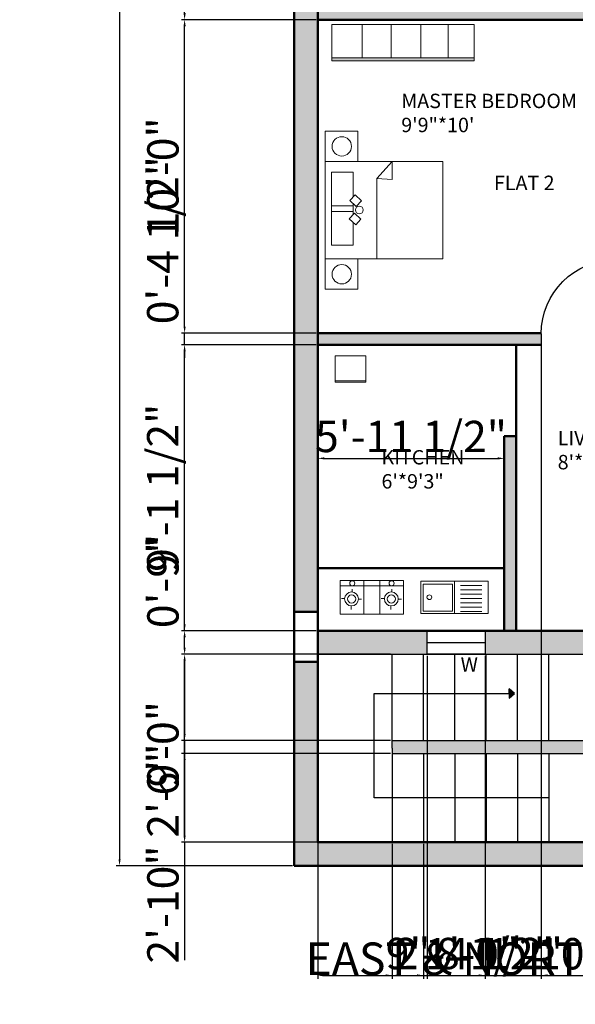
# Model space of a CAD drawing. Units: inches. Extents: x 2063 to 3370, y 2091 to 2971.
# Tile 3 of 14: x 2498 to 2710, y 2091 to 2468. Entities that reach past the tile are written whole.
import ezdxf

# ---------------------------------------------------------------- set-up
doc = ezdxf.new("R2010")
doc.units = ezdxf.units.IN
for name, color, linetype, lineweight in [('A-ANNO-DIMS', 2, 'Continuous', 18), ('A-ANNO-TEXT', 7, 'Continuous', 18), ('A-AREA-IDEN', 3, 'Continuous', 18), ('A-COLS', 7, 'Continuous', 50), ('A-DOOR', 4, 'Continuous', 25), ('A-EQPM', 8, 'Continuous', 18), ('A-FLOR-FIXT', 9, 'Continuous', 18), ('A-FLOR-STRS', 3, 'Continuous', 25), ('A-FURN', 8, 'Continuous', 18), ('A-GLAZ', 131, 'Continuous', 25), ('A-WALL', 7, 'Continuous', 50), ('A-WALL-PATT', 8, 'Continuous', 13)]:
    doc.layers.add(name, color=color, linetype=linetype, lineweight=lineweight)
doc.styles.get("Standard").update_dxf_attribs({"font": 'arial.ttf'})
doc.dimstyles.new('ISO-25', dxfattribs={"dimtxt": 12, "dimasz": 2.5, "dimexe": 1.25, "dimexo": 0.625, "dimtad": 1, "dimdec": 0, "dimlunit": 4, "dimtxsty": 'Standard', "dimcen": 2.5, "dimadec": 0, "dimazin": 0, "dimtfac": 1, "dimtdec": 0, "dimtmove": 0, "dimatfit": 3, "dimfxl": 1, "dimarcsym": 0})

# ---------------------------------------------------------------- blocks, each defined once
blk = doc.blocks.new('*D8')
at = {"layer": 'A-ANNO-DIMS', "color": 0, "lineweight": -2, "transparency": 16777216}
for p, q in [((2602.12, 2864.43), (2534.59, 2864.43)), ((2535.84, 2861.93), (2535.84, 2146.93)), ((2602.12, 2144.43), (2534.59, 2144.43))]:
    blk.add_line(p, q, dxfattribs=at)
at = {"layer": 'A-ANNO-DIMS', "color": 0, "transparency": 16777216}
for points in [[(2535.42, 2861.93), (2536.25, 2861.93), (2535.84, 2864.43)], [(2535.42, 2146.93), (2536.25, 2146.93), (2535.84, 2144.43)]]:
    blk.add_solid(points, dxfattribs=at)
at = {"layer": 'Defpoints', "color": 0, "transparency": 16777216}
for p in [(2602.75, 2864.43), (2535.84, 2144.43), (2602.75, 2144.43)]:
    blk.add_point(p, dxfattribs=at)
at = {"layer": 'A-ANNO-DIMS', "color": 0, "transparency": 16777216, "insert": (2529.08, 2504.43), "char_height": 12, "attachment_point": 5, "rotation": 90}
blk.add_mtext("60'", dxfattribs=at)
blk = doc.blocks.new('*U2')
for p, q in [((0, 0), (0, -6)), ((40, 0), (40, -6))]:
    blk.add_line(p, q)
blk.add_lwpolyline([(0, 0), (0, 40), (1.75, 40), (1.75, 0)], close=True)
blk.add_arc((0, 0), 40, 0, 90)
blk = doc.blocks.new('SINK')
for p, q in [((12.88, 12.38), (12.88, 0)), ((15.15, 10.72), (23.41, 10.72)), ((15.15, 9.06), (23.41, 9.06)), ((15.15, 7.39), (23.41, 7.39)), ((15.15, 5.73), (23.41, 5.73)), ((15.15, 4.07), (23.41, 4.07)), ((15.15, 2.41), (23.41, 2.41)), ((15.15, 0.75), (23.41, 0.75))]:
    blk.add_line(p, q)
for points in [[(25.76, 12.38), (0, 12.38), (0, 0), (25.76, 0)], [(0.92, 11.24), (12.1, 11.24), (12.1, 0.97), (0.92, 0.97)]]:
    blk.add_lwpolyline(points, close=True)
blk.add_circle((3.27, 6.25), 0.918)
blk = doc.blocks.new('STOVE')
for p, q in [((0, 12.93), (9.11, 12.93)), ((9.11, 12.93), (9.11, 0)), ((15.17, 0), (15.17, 12.93)), ((0, 10.85), (24.22, 10.85)), ((4.55, 8.54), (4.55, 9.68)), ((19.76, 8.54), (19.76, 9.68)), ((1.72, 5.99), (0.55, 5.99)), ((7.04, 5.79), (8.23, 5.79)), ((16.93, 5.99), (15.75, 5.99)), ((22.25, 5.79), (23.43, 5.79)), ((4.22, 3.16), (4.22, 1.87)), ((24.22, 0), (15.17, 0)), ((19.43, 3.16), (19.43, 1.87))]:
    blk.add_line(p, q)
blk.add_lwpolyline([(0, 12.93), (24.22, 12.93), (24.22, 0), (0, 0)], close=True)
for centre, radius in [((4.62, 11.87), 0.973), ((19.71, 11.87), 0.973), ((4.38, 5.88), 2.66), ((19.59, 5.88), 2.66), ((4.38, 5.88), 1.57), ((19.59, 5.88), 1.57)]:
    blk.add_circle(centre, radius)
blk = doc.blocks.new('*D28')
at = {"layer": 'A-ANNO-DIMS', "color": 0, "lineweight": -2, "transparency": 16777216}
for p, q in [((2647.53, 2480.55), (2647.53, 2476.06)), ((2673.28, 2480.55), (2673.28, 2476.06)), ((2650.03, 2477.31), (2670.78, 2477.31)), ((2673.28, 2477.31), (2793.91, 2477.31))]:
    blk.add_line(p, q, dxfattribs=at)
at = {"layer": 'A-ANNO-DIMS', "color": 0, "transparency": 16777216}
for points in [[(2650.03, 2477.73), (2650.03, 2476.9), (2647.53, 2477.31)], [(2670.78, 2477.73), (2670.78, 2476.9), (2673.28, 2477.31)]]:
    blk.add_solid(points, dxfattribs=at)
at = {"layer": 'Defpoints', "color": 0, "transparency": 16777216}
for p in [(2647.53, 2481.18), (2673.28, 2481.18), (2673.28, 2477.31)]:
    blk.add_point(p, dxfattribs=at)
at = {"layer": 'A-ANNO-DIMS', "color": 0, "transparency": 16777216, "insert": (2734.85, 2484.14), "char_height": 12, "attachment_point": 5}
blk.add_mtext('SINK 2\'-2" TYP.', dxfattribs=at)
blk = doc.blocks.new('*D88')
at = {"layer": 'A-ANNO-DIMS', "color": 0, "lineweight": -2, "transparency": 16777216}
for p, q in [((2611.75, 2152.8), (2611.75, 2101.18)), ((2640.25, 2152.8), (2640.25, 2101.18)), ((2614.25, 2102.43), (2637.75, 2102.43)), ((2640.25, 2102.43), (2704.06, 2102.43))]:
    blk.add_line(p, q, dxfattribs=at)
at = {"layer": 'A-ANNO-DIMS', "color": 0, "transparency": 16777216}
for points in [[(2614.25, 2102.84), (2614.25, 2102.01), (2611.75, 2102.43)], [(2637.75, 2102.84), (2637.75, 2102.01), (2640.25, 2102.43)]]:
    blk.add_solid(points, dxfattribs=at)
at = {"layer": 'Defpoints', "color": 0, "transparency": 16777216}
for p in [(2611.75, 2153.43), (2640.25, 2153.43), (2640.25, 2102.43)]:
    blk.add_point(p, dxfattribs=at)
at = {"layer": 'A-ANNO-DIMS', "color": 0, "transparency": 16777216, "insert": (2673.4, 2109.26), "char_height": 12, "attachment_point": 5}
blk.add_mtext('2\'-4 1/2"', dxfattribs=at)
blk = doc.blocks.new('*D89')
at = {"layer": 'A-ANNO-DIMS', "color": 0, "lineweight": -2, "transparency": 16777216}
for p, q in [((2640.25, 2152.8), (2640.25, 2101.18)), ((2652.25, 2152.8), (2652.25, 2101.18)), ((2642.75, 2102.43), (2649.75, 2102.43)), ((2652.25, 2102.43), (2686.77, 2102.43))]:
    blk.add_line(p, q, dxfattribs=at)
at = {"layer": 'A-ANNO-DIMS', "color": 0, "transparency": 16777216}
for points in [[(2642.75, 2102.84), (2642.75, 2102.01), (2640.25, 2102.43)], [(2649.75, 2102.84), (2649.75, 2102.01), (2652.25, 2102.43)]]:
    blk.add_solid(points, dxfattribs=at)
at = {"layer": 'Defpoints', "color": 0, "transparency": 16777216}
for p in [(2640.25, 2153.43), (2652.25, 2153.43), (2652.25, 2102.43)]:
    blk.add_point(p, dxfattribs=at)
at = {"layer": 'A-ANNO-DIMS', "color": 0, "transparency": 16777216, "insert": (2670.76, 2109.18), "char_height": 12, "attachment_point": 5}
blk.add_mtext('1\'-0"', dxfattribs=at)
blk = doc.blocks.new('*D90')
at = {"layer": 'A-ANNO-DIMS', "color": 0, "lineweight": -2, "transparency": 16777216}
for p, q in [((2653.66, 2224.8), (2653.66, 2101.18)), ((2675.81, 2224.8), (2675.81, 2101.18)), ((2656.16, 2102.43), (2673.31, 2102.43)), ((2675.81, 2102.43), (2719.66, 2102.43))]:
    blk.add_line(p, q, dxfattribs=at)
at = {"layer": 'A-ANNO-DIMS', "color": 0, "transparency": 16777216}
for points in [[(2656.16, 2102.84), (2656.16, 2102.01), (2653.66, 2102.43)], [(2673.31, 2102.84), (2673.31, 2102.01), (2675.81, 2102.43)]]:
    blk.add_solid(points, dxfattribs=at)
at = {"layer": 'Defpoints', "color": 0, "transparency": 16777216}
for p in [(2653.66, 2225.43), (2675.81, 2225.43), (2675.81, 2102.43)]:
    blk.add_point(p, dxfattribs=at)
at = {"layer": 'A-ANNO-DIMS', "color": 0, "transparency": 16777216, "insert": (2698.99, 2109.18), "char_height": 12, "attachment_point": 5}
blk.add_mtext('1\'-10"', dxfattribs=at)
blk = doc.blocks.new('*D92')
at = {"layer": 'A-ANNO-DIMS', "color": 0, "lineweight": -2, "transparency": 16777216}
for p, q in [((2611.75, 2259.05), (2611.75, 2301.68)), ((2614.25, 2300.43), (2680.64, 2300.43)), ((2683.14, 2259.05), (2683.14, 2301.68))]:
    blk.add_line(p, q, dxfattribs=at)
at = {"layer": 'A-ANNO-DIMS', "color": 0, "transparency": 16777216}
for points in [[(2614.25, 2300.84), (2614.25, 2300.01), (2611.75, 2300.43)], [(2680.64, 2300.84), (2680.64, 2300.01), (2683.14, 2300.43)]]:
    blk.add_solid(points, dxfattribs=at)
at = {"layer": 'Defpoints', "color": 0, "transparency": 16777216}
for p in [(2683.14, 2300.43), (2611.75, 2258.43), (2683.14, 2258.43)]:
    blk.add_point(p, dxfattribs=at)
at = {"layer": 'A-ANNO-DIMS', "color": 0, "transparency": 16777216, "insert": (2647.44, 2307.26), "char_height": 12, "attachment_point": 5}
blk.add_mtext('5\'-11 1/2"', dxfattribs=at)
blk = doc.blocks.new('*D94')
at = {"layer": 'A-ANNO-DIMS', "color": 0, "lineweight": -2, "transparency": 16777216}
for p, q in [((2611.75, 2347.8), (2611.75, 2101.18)), ((2728.14, 2347.8), (2728.14, 2101.18)), ((2614.25, 2102.43), (2725.64, 2102.43))]:
    blk.add_line(p, q, dxfattribs=at)
at = {"layer": 'A-ANNO-DIMS', "color": 0, "transparency": 16777216}
for points in [[(2614.25, 2102.84), (2614.25, 2102.01), (2611.75, 2102.43)], [(2725.64, 2102.84), (2725.64, 2102.01), (2728.14, 2102.43)]]:
    blk.add_solid(points, dxfattribs=at)
at = {"layer": 'Defpoints', "color": 0, "transparency": 16777216}
for p in [(2611.75, 2348.43), (2728.14, 2348.43), (2728.14, 2102.43)]:
    blk.add_point(p, dxfattribs=at)
at = {"layer": 'A-ANNO-DIMS', "color": 0, "transparency": 16777216, "insert": (2669.94, 2109.26), "char_height": 12, "attachment_point": 5}
blk.add_mtext('9\'-8 1/2"', dxfattribs=at)
blk = doc.blocks.new('*D98')
at = {"layer": 'A-ANNO-DIMS', "color": 0, "lineweight": -2, "transparency": 16777216}
for p, q in [((2611.12, 2225.43), (2559.5, 2225.43)), ((2560.75, 2155.93), (2560.75, 2222.93)), ((2611.12, 2153.43), (2559.5, 2153.43))]:
    blk.add_line(p, q, dxfattribs=at)
at = {"layer": 'A-ANNO-DIMS', "color": 0, "transparency": 16777216}
for points in [[(2560.33, 2222.93), (2561.16, 2222.93), (2560.75, 2225.43)], [(2560.33, 2155.93), (2561.16, 2155.93), (2560.75, 2153.43)]]:
    blk.add_solid(points, dxfattribs=at)
at = {"layer": 'Defpoints', "color": 0, "transparency": 16777216}
for p in [(2560.75, 2225.43), (2611.75, 2225.43), (2611.75, 2153.43)]:
    blk.add_point(p, dxfattribs=at)
at = {"layer": 'A-ANNO-DIMS', "color": 0, "transparency": 16777216, "insert": (2554, 2189.43), "char_height": 12, "attachment_point": 5, "rotation": 90}
blk.add_mtext('6\'-0"', dxfattribs=at)
blk = doc.blocks.new('*D99')
at = {"layer": 'A-ANNO-DIMS', "color": 0, "lineweight": -2, "transparency": 16777216}
for p, q in [((2560.75, 2234.43), (2560.75, 2270.08)), ((2611.12, 2234.43), (2559.5, 2234.43)), ((2560.75, 2227.93), (2560.75, 2231.93)), ((2611.12, 2225.43), (2559.5, 2225.43))]:
    blk.add_line(p, q, dxfattribs=at)
at = {"layer": 'A-ANNO-DIMS', "color": 0, "transparency": 16777216}
for points in [[(2560.33, 2231.93), (2561.16, 2231.93), (2560.75, 2234.43)], [(2560.33, 2227.93), (2561.16, 2227.93), (2560.75, 2225.43)]]:
    blk.add_solid(points, dxfattribs=at)
at = {"layer": 'Defpoints', "color": 0, "transparency": 16777216}
for p in [(2560.75, 2234.43), (2611.75, 2234.43), (2611.75, 2225.43)]:
    blk.add_point(p, dxfattribs=at)
at = {"layer": 'A-ANNO-DIMS', "color": 0, "transparency": 16777216, "insert": (2554, 2253.5), "char_height": 12, "attachment_point": 5, "rotation": 90}
blk.add_mtext('0\'-9"', dxfattribs=at)
blk = doc.blocks.new('*D100')
at = {"layer": 'A-ANNO-DIMS', "color": 0, "lineweight": -2, "transparency": 16777216}
for p, q in [((2611.12, 2343.93), (2559.5, 2343.93)), ((2560.75, 2236.93), (2560.75, 2341.43)), ((2611.12, 2234.43), (2559.5, 2234.43))]:
    blk.add_line(p, q, dxfattribs=at)
at = {"layer": 'A-ANNO-DIMS', "color": 0, "transparency": 16777216}
for points in [[(2560.33, 2341.43), (2561.16, 2341.43), (2560.75, 2343.93)], [(2560.33, 2236.93), (2561.16, 2236.93), (2560.75, 2234.43)]]:
    blk.add_solid(points, dxfattribs=at)
at = {"layer": 'Defpoints', "color": 0, "transparency": 16777216}
for p in [(2560.75, 2343.93), (2611.75, 2343.93), (2611.75, 2234.43)]:
    blk.add_point(p, dxfattribs=at)
at = {"layer": 'A-ANNO-DIMS', "color": 0, "transparency": 16777216, "insert": (2553.92, 2289.18), "char_height": 12, "attachment_point": 5, "rotation": 90}
blk.add_mtext('9\'-1 1/2"', dxfattribs=at)
blk = doc.blocks.new('*D101')
at = {"layer": 'A-ANNO-DIMS', "color": 0, "lineweight": -2, "transparency": 16777216}
for p, q in [((2560.75, 2350.93), (2560.75, 2414.54)), ((2611.12, 2348.43), (2559.5, 2348.43)), ((2560.75, 2343.93), (2560.75, 2348.43)), ((2611.12, 2343.93), (2559.5, 2343.93)), ((2560.75, 2341.43), (2560.75, 2338.93))]:
    blk.add_line(p, q, dxfattribs=at)
at = {"layer": 'A-ANNO-DIMS', "color": 0, "transparency": 16777216}
for points in [[(2560.33, 2350.93), (2561.16, 2350.93), (2560.75, 2348.43)], [(2560.33, 2341.43), (2561.16, 2341.43), (2560.75, 2343.93)]]:
    blk.add_solid(points, dxfattribs=at)
at = {"layer": 'Defpoints', "color": 0, "transparency": 16777216}
for p in [(2560.75, 2348.43), (2611.75, 2348.43), (2611.75, 2343.93)]:
    blk.add_point(p, dxfattribs=at)
at = {"layer": 'A-ANNO-DIMS', "color": 0, "transparency": 16777216, "insert": (2553.92, 2383.98), "char_height": 12, "attachment_point": 5, "rotation": 90}
blk.add_mtext('0\'-4 1/2"', dxfattribs=at)
blk = doc.blocks.new('*D102')
at = {"layer": 'A-ANNO-DIMS', "color": 0, "lineweight": -2, "transparency": 16777216}
for p, q in [((2611.12, 2468.43), (2559.5, 2468.43)), ((2560.75, 2350.93), (2560.75, 2465.93)), ((2611.12, 2348.43), (2559.5, 2348.43))]:
    blk.add_line(p, q, dxfattribs=at)
at = {"layer": 'A-ANNO-DIMS', "color": 0, "transparency": 16777216}
for points in [[(2560.33, 2465.93), (2561.16, 2465.93), (2560.75, 2468.43)], [(2560.33, 2350.93), (2561.16, 2350.93), (2560.75, 2348.43)]]:
    blk.add_solid(points, dxfattribs=at)
at = {"layer": 'Defpoints', "color": 0, "transparency": 16777216}
for p in [(2560.75, 2468.43), (2611.75, 2468.43), (2611.75, 2348.43)]:
    blk.add_point(p, dxfattribs=at)
at = {"layer": 'A-ANNO-DIMS', "color": 0, "transparency": 16777216, "insert": (2554, 2408.43), "char_height": 12, "attachment_point": 5, "rotation": 90}
blk.add_mtext('10\'-0"', dxfattribs=at)
blk = doc.blocks.new('*D103')
at = {"layer": 'A-ANNO-DIMS', "color": 0, "lineweight": -2, "transparency": 16777216}
for p, q in [((2560.75, 2477.43), (2560.75, 2513.08)), ((2611.12, 2477.43), (2559.5, 2477.43)), ((2560.75, 2470.93), (2560.75, 2474.93)), ((2611.12, 2468.43), (2559.5, 2468.43))]:
    blk.add_line(p, q, dxfattribs=at)
at = {"layer": 'A-ANNO-DIMS', "color": 0, "transparency": 16777216}
for points in [[(2560.33, 2474.93), (2561.16, 2474.93), (2560.75, 2477.43)], [(2560.33, 2470.93), (2561.16, 2470.93), (2560.75, 2468.43)]]:
    blk.add_solid(points, dxfattribs=at)
at = {"layer": 'Defpoints', "color": 0, "transparency": 16777216}
for p in [(2560.75, 2477.43), (2611.75, 2477.43), (2611.75, 2468.43)]:
    blk.add_point(p, dxfattribs=at)
at = {"layer": 'A-ANNO-DIMS', "color": 0, "transparency": 16777216, "insert": (2554, 2496.5), "char_height": 12, "attachment_point": 5, "rotation": 90}
blk.add_mtext('0\'-9"', dxfattribs=at)
blk = doc.blocks.new('*D126')
at = {"layer": 'A-ANNO-DIMS', "color": 0, "lineweight": -2, "transparency": 16777216}
for p, q in [((2639.62, 2225.43), (2559.5, 2225.43)), ((2560.75, 2222.93), (2560.75, 2194.93)), ((2639.62, 2192.43), (2559.5, 2192.43)), ((2560.75, 2192.43), (2560.75, 2156.57))]:
    blk.add_line(p, q, dxfattribs=at)
at = {"layer": 'A-ANNO-DIMS', "color": 0, "transparency": 16777216}
for points in [[(2560.33, 2222.93), (2561.16, 2222.93), (2560.75, 2225.43)], [(2560.33, 2194.93), (2561.16, 2194.93), (2560.75, 2192.43)]]:
    blk.add_solid(points, dxfattribs=at)
at = {"layer": 'Defpoints', "color": 0, "transparency": 16777216}
for p in [(2640.25, 2225.43), (2560.75, 2192.43), (2640.25, 2192.43)]:
    blk.add_point(p, dxfattribs=at)
at = {"layer": 'A-ANNO-DIMS', "color": 0, "transparency": 16777216, "insert": (2554, 2173.25), "char_height": 12, "attachment_point": 5, "rotation": 90}
blk.add_mtext('2\'-9"', dxfattribs=at)
blk = doc.blocks.new('*D127')
at = {"layer": 'A-ANNO-DIMS', "color": 0, "lineweight": -2, "transparency": 16777216}
for p, q in [((2639.62, 2187.43), (2559.5, 2187.43)), ((2560.75, 2184.93), (2560.75, 2155.93)), ((2639.62, 2153.43), (2559.5, 2153.43)), ((2560.75, 2153.43), (2560.75, 2108.25))]:
    blk.add_line(p, q, dxfattribs=at)
at = {"layer": 'A-ANNO-DIMS', "color": 0, "transparency": 16777216}
for points in [[(2560.33, 2184.93), (2561.16, 2184.93), (2560.75, 2187.43)], [(2560.33, 2155.93), (2561.16, 2155.93), (2560.75, 2153.43)]]:
    blk.add_solid(points, dxfattribs=at)
at = {"layer": 'Defpoints', "color": 0, "transparency": 16777216}
for p in [(2640.25, 2187.43), (2560.75, 2153.43), (2640.25, 2153.43)]:
    blk.add_point(p, dxfattribs=at)
at = {"layer": 'A-ANNO-DIMS', "color": 0, "transparency": 16777216, "insert": (2554, 2129.59), "char_height": 12, "attachment_point": 5, "rotation": 90}
blk.add_mtext('2\'-10"', dxfattribs=at)
blk = doc.blocks.new('*D132')
at = {"layer": 'A-ANNO-DIMS', "color": 0, "lineweight": -2, "transparency": 16777216}
for p, q in [((2697.29, 2347.55), (2697.29, 2101.18)), ((2725.61, 2347.55), (2725.61, 2101.18)), ((2699.79, 2102.43), (2723.11, 2102.43)), ((2725.61, 2102.43), (2789.42, 2102.43))]:
    blk.add_line(p, q, dxfattribs=at)
at = {"layer": 'A-ANNO-DIMS', "color": 0, "transparency": 16777216}
for points in [[(2699.79, 2102.84), (2699.79, 2102.01), (2697.29, 2102.43)], [(2723.11, 2102.84), (2723.11, 2102.01), (2725.61, 2102.43)]]:
    blk.add_solid(points, dxfattribs=at)
at = {"layer": 'Defpoints', "color": 0, "transparency": 16777216}
for p in [(2697.29, 2348.17), (2725.61, 2348.17), (2725.61, 2102.43)]:
    blk.add_point(p, dxfattribs=at)
at = {"layer": 'A-ANNO-DIMS', "color": 0, "transparency": 16777216, "insert": (2758.77, 2109.26), "char_height": 12, "attachment_point": 5}
blk.add_mtext('2\'-4 1/2"', dxfattribs=at)

msp = doc.modelspace()

# ---------------------------------------------------------------- hatches: boundary and pattern name
at = {"layer": 'A-FLOR-STRS'}
h = msp.add_hatch(color=256, dxfattribs=at)
h.dxf.hatch_style = 1
h.paths.add_polyline_path([(2687.09, 2210.45), (2685.01, 2212.18), (2685.01, 2210.45), (2685.01, 2208.56)])
at = {"layer": 'A-FURN'}
h = msp.add_hatch(color=256, dxfattribs=at)
h.dxf.hatch_style = 1
h.paths.add_polyline_path([(2671.63, 2452.62), (2671.63, 2453.88), (2617.14, 2453.8), (2617.14, 2452.62)])
at = {"layer": 'A-WALL-PATT'}
h = msp.add_hatch(color=256, dxfattribs=at)
h.dxf.hatch_style = 1
h.paths.add_polyline_path([(2842.75, 2864.43), (2602.75, 2864.43), (2602.75, 2831.43), (2608.62, 2831.43), (2608.62, 2859.54), (2836.36, 2859.54), (2836.36, 2831.15), (2842.75, 2831.15)])
h.paths.add_polyline_path([(2775.49, 2177.04), (2815.13, 2177.04), (2815.13, 2197.65), (2775.49, 2197.65)], flags=9)
h.paths.add_polyline_path([(2634.18, 2285.75), (2670.81, 2285.75), (2670.81, 2306.35), (2634.18, 2306.35)], flags=9)
h.paths.add_polyline_path([(2701.65, 2293.1), (2755.85, 2293.1), (2755.85, 2313.71), (2701.65, 2313.71)], flags=9)
h.paths.add_polyline_path([(2735.8, 2415.55), (2772.95, 2415.55), (2772.95, 2436.13), (2735.8, 2436.13)], flags=9)
h.paths.add_polyline_path([(2641.75, 2422.21), (2718.67, 2422.21), (2718.67, 2442.82), (2641.75, 2442.82)], flags=9)
h.paths.add_polyline_path([(2710.43, 2552.92), (2764.91, 2552.92), (2764.91, 2573.53), (2710.43, 2573.53)], flags=9)
h.paths.add_polyline_path([(2625.23, 2527.83), (2661.86, 2527.83), (2661.86, 2548.44), (2625.23, 2548.44)], flags=9)
h.paths.add_polyline_path([(2627.53, 2598.16), (2652.13, 2598.16), (2652.13, 2618.77), (2627.53, 2618.77)], flags=9)
h.paths.add_polyline_path([(2646.64, 2696.08), (2723.56, 2696.08), (2723.56, 2716.69), (2646.64, 2716.69)], flags=9)
h.paths.add_polyline_path([(2791.65, 2795.64), (2828.72, 2795.64), (2828.72, 2807.02), (2791.65, 2807.02)], flags=9)
h.paths.add_polyline_path([(2751.88, 2214.78), (2761.93, 2214.78), (2761.93, 2226.17), (2751.88, 2226.17)], flags=9)
h.paths.add_polyline_path([(2664.96, 2215.71), (2675, 2215.71), (2675, 2227.09), (2664.96, 2227.09)], flags=9)
h.paths.add_polyline_path([(2788.26, 2413.43), (2796.17, 2413.43), (2796.17, 2424.82), (2788.26, 2424.82)], flags=9)
h.paths.add_polyline_path([(2728.86, 2795.64), (2765.93, 2795.64), (2765.93, 2807.02), (2728.86, 2807.02)], flags=9)
h.paths.add_polyline_path([(2760.39, 2726.09), (2823.16, 2726.09), (2823.16, 2746.7), (2760.39, 2746.7)], flags=9)
h = msp.add_hatch(color=256, dxfattribs=at)
h.dxf.hatch_style = 1
h.paths.add_polyline_path([(2290.22, 2192.43), (2278.22, 2192.43), (2182.22, 2192.43), (2182.22, 2189.43), (2182.22, 2187.43), (2278.22, 2187.43), (2290.22, 2187.42)])
h.paths.add_polyline_path([(2748.25, 2192.43), (2736.25, 2192.43), (2640.25, 2192.43), (2640.25, 2189.43), (2640.25, 2187.43), (2736.25, 2187.43), (2748.25, 2187.42)], flags=17)
h.paths.add_polyline_path([(2653.66, 2234.43), (2611.75, 2234.43), (2611.75, 2232.93), (2611.75, 2225.43), (2653.66, 2225.43)])
h.paths.add_polyline_path([(2717.13, 2234.43), (2675.81, 2234.43), (2675.81, 2225.43), (2717.13, 2225.43)])
h.paths.add_polyline_path([(2611.75, 2222.57), (2602.75, 2222.57), (2602.75, 2144.43), (2842.75, 2144.43), (2842.75, 2220.3), (2833.75, 2220.3), (2833.75, 2153.43), (2829.39, 2153.43), (2754.78, 2153.43), (2611.75, 2153.43)])
h.paths.add_polyline_path([(2687.64, 2308.91), (2683.14, 2308.91), (2683.14, 2234.43), (2687.64, 2234.43)])
h.paths.add_polyline_path([(2744.5, 2234.43), (2736.25, 2234.43), (2736.25, 2225.43), (2744.5, 2225.43)])
h.paths.add_polyline_path([(2785.14, 2260.02), (2782.31, 2260.02), (2780.64, 2260.02), (2780.64, 2234.43), (2766.65, 2234.43), (2766.65, 2225.43), (2785.14, 2225.43)])
h.paths.add_polyline_path([(2842.75, 2363.93), (2833.75, 2363.93), (2833.75, 2239.41), (2842.75, 2239.41)])
h.paths.add_polyline_path([(2775.49, 2177.04), (2815.13, 2177.04), (2815.13, 2197.65), (2775.49, 2197.65)], flags=25)
h.paths.add_polyline_path([(2634.18, 2285.75), (2670.81, 2285.75), (2670.81, 2306.35), (2634.18, 2306.35)], flags=9)
h.paths.add_polyline_path([(2701.65, 2293.1), (2755.85, 2293.1), (2755.85, 2313.71), (2701.65, 2313.71)], flags=9)
h.paths.add_polyline_path([(2735.8, 2415.55), (2772.95, 2415.55), (2772.95, 2436.13), (2735.8, 2436.13)], flags=9)
h.paths.add_polyline_path([(2641.75, 2422.21), (2718.67, 2422.21), (2718.67, 2442.82), (2641.75, 2442.82)], flags=9)
h.paths.add_polyline_path([(2710.43, 2552.92), (2764.91, 2552.92), (2764.91, 2573.53), (2710.43, 2573.53)], flags=9)
h.paths.add_polyline_path([(2625.23, 2527.83), (2661.86, 2527.83), (2661.86, 2548.44), (2625.23, 2548.44)], flags=9)
h.paths.add_polyline_path([(2627.53, 2598.16), (2652.13, 2598.16), (2652.13, 2618.77), (2627.53, 2618.77)], flags=9)
h.paths.add_polyline_path([(2646.64, 2696.08), (2723.56, 2696.08), (2723.56, 2716.69), (2646.64, 2716.69)], flags=9)
h.paths.add_polyline_path([(2791.65, 2795.64), (2828.72, 2795.64), (2828.72, 2807.02), (2791.65, 2807.02)], flags=9)
h.paths.add_polyline_path([(2751.88, 2214.78), (2761.93, 2214.78), (2761.93, 2226.17), (2751.88, 2226.17)], flags=9)
h.paths.add_polyline_path([(2788.26, 2413.43), (2796.17, 2413.43), (2796.17, 2424.82), (2788.26, 2424.82)], flags=9)
h.paths.add_polyline_path([(2761.97, 2835.24), (2769.88, 2835.24), (2769.88, 2846.62), (2761.97, 2846.62)], flags=9)
h.paths.add_polyline_path([(2675.89, 2833.68), (2685.93, 2833.68), (2685.93, 2845.06), (2675.89, 2845.06)], flags=9)
h.paths.add_polyline_path([(2728.86, 2795.64), (2765.93, 2795.64), (2765.93, 2807.02), (2728.86, 2807.02)], flags=9)
h.paths.add_polyline_path([(2760.39, 2726.09), (2823.16, 2726.09), (2823.16, 2746.7), (2760.39, 2746.7)], flags=9)
h = msp.add_hatch(color=256, dxfattribs=at)
h.dxf.hatch_style = 1
h.paths.add_polyline_path([(2680.75, 2631.93), (2684.44, 2631.93), (2684.44, 2636.43), (2683.1, 2636.43), (2611.75, 2636.43), (2611.75, 2631.93), (2648.72, 2631.93), (2671.75, 2631.93), (2676.25, 2631.93), (2676.25, 2623.58), (2678.23, 2623.58), (2680.75, 2623.58)])
h.paths.add_polyline_path([(2728.75, 2636.43), (2724.44, 2636.43), (2724.44, 2631.93), (2728.75, 2631.93)])
h.paths.add_polyline_path([(2772.02, 2636.43), (2733.25, 2636.43), (2733.25, 2631.93), (2772.02, 2631.93)])
h.paths.add_polyline_path([(2733.25, 2636.43), (2728.75, 2636.43), (2728.75, 2631.93), (2733.25, 2631.93)])
h.paths.add_polyline_path([(2833.75, 2636.43), (2812.02, 2636.43), (2812.02, 2631.93), (2833.75, 2631.93)])
h.paths.add_polyline_path([(2842.75, 2626.16), (2833.75, 2626.16), (2833.75, 2585.28), (2842.75, 2585.28)])
h.paths.add_polyline_path([(2842.75, 2679.03), (2833.75, 2679.03), (2833.75, 2645.28), (2842.75, 2645.28)])
h.paths.add_polyline_path([(2611.75, 2619.52), (2602.75, 2619.52), (2602.75, 2548.5), (2611.75, 2548.5), (2611.75, 2579.43)])
h.paths.add_polyline_path([(2646.64, 2696.08), (2723.56, 2696.08), (2723.56, 2716.69), (2646.64, 2716.69)], flags=9)
h.paths.add_polyline_path([(2791.65, 2795.64), (2828.72, 2795.64), (2828.72, 2807.02), (2791.65, 2807.02)], flags=9)
h.paths.add_polyline_path([(2761.97, 2835.24), (2769.88, 2835.24), (2769.88, 2846.62), (2761.97, 2846.62)], flags=9)
h.paths.add_polyline_path([(2675.89, 2833.68), (2685.93, 2833.68), (2685.93, 2845.06), (2675.89, 2845.06)], flags=9)
h.paths.add_polyline_path([(2728.86, 2795.64), (2765.93, 2795.64), (2765.93, 2807.02), (2728.86, 2807.02)], flags=9)
h.paths.add_polyline_path([(2775.49, 2177.04), (2815.13, 2177.04), (2815.13, 2197.65), (2775.49, 2197.65)], flags=9)
h.paths.add_polyline_path([(2634.18, 2285.75), (2670.81, 2285.75), (2670.81, 2306.35), (2634.18, 2306.35)], flags=9)
h.paths.add_polyline_path([(2701.65, 2293.1), (2755.85, 2293.1), (2755.85, 2313.71), (2701.65, 2313.71)], flags=9)
h.paths.add_polyline_path([(2735.8, 2415.55), (2772.95, 2415.55), (2772.95, 2436.13), (2735.8, 2436.13)], flags=9)
h.paths.add_polyline_path([(2641.75, 2422.21), (2718.67, 2422.21), (2718.67, 2442.82), (2641.75, 2442.82)], flags=9)
h.paths.add_polyline_path([(2710.43, 2552.92), (2764.91, 2552.92), (2764.91, 2573.53), (2710.43, 2573.53)], flags=9)
h.paths.add_polyline_path([(2625.23, 2527.83), (2661.86, 2527.83), (2661.86, 2548.44), (2625.23, 2548.44)], flags=9)
h.paths.add_polyline_path([(2751.88, 2214.78), (2761.93, 2214.78), (2761.93, 2226.17), (2751.88, 2226.17)], flags=9)
h.paths.add_polyline_path([(2664.96, 2215.71), (2675, 2215.71), (2675, 2227.09), (2664.96, 2227.09)], flags=9)
h.paths.add_polyline_path([(2788.26, 2413.43), (2796.17, 2413.43), (2796.17, 2424.82), (2788.26, 2424.82)], flags=9)
h = msp.add_hatch(color=256, dxfattribs=at)
h.dxf.hatch_style = 1
h.paths.add_polyline_path([(2611.75, 2343.93), (2611.75, 2477.43), (2611.75, 2514.15), (2602.75, 2514.15), (2602.75, 2241.68), (2611.75, 2241.68), (2611.75, 2258.43)])
h.paths.add_polyline_path([(2775.49, 2177.04), (2815.13, 2177.04), (2815.13, 2197.65), (2775.49, 2197.65)], flags=9)
h.paths.add_polyline_path([(2735.8, 2415.55), (2772.95, 2415.55), (2772.95, 2436.13), (2735.8, 2436.13)], flags=9)
h.paths.add_polyline_path([(2641.75, 2422.21), (2718.67, 2422.21), (2718.67, 2442.82), (2641.75, 2442.82)], flags=9)
h.paths.add_polyline_path([(2710.43, 2552.92), (2764.91, 2552.92), (2764.91, 2573.53), (2710.43, 2573.53)], flags=9)
h.paths.add_polyline_path([(2625.23, 2527.83), (2661.86, 2527.83), (2661.86, 2548.44), (2625.23, 2548.44)], flags=9)
h.paths.add_polyline_path([(2627.53, 2598.16), (2652.13, 2598.16), (2652.13, 2618.77), (2627.53, 2618.77)], flags=9)
h.paths.add_polyline_path([(2646.64, 2696.08), (2723.56, 2696.08), (2723.56, 2716.69), (2646.64, 2716.69)], flags=9)
h.paths.add_polyline_path([(2791.65, 2795.64), (2828.72, 2795.64), (2828.72, 2807.02), (2791.65, 2807.02)], flags=9)
h.paths.add_polyline_path([(2751.88, 2214.78), (2761.93, 2214.78), (2761.93, 2226.17), (2751.88, 2226.17)], flags=9)
h.paths.add_polyline_path([(2788.26, 2413.43), (2796.17, 2413.43), (2796.17, 2424.82), (2788.26, 2424.82)], flags=9)
h.paths.add_polyline_path([(2761.97, 2835.24), (2769.88, 2835.24), (2769.88, 2846.62), (2761.97, 2846.62)], flags=9)
h.paths.add_polyline_path([(2675.89, 2833.68), (2685.93, 2833.68), (2685.93, 2845.06), (2675.89, 2845.06)], flags=9)
h.paths.add_polyline_path([(2728.86, 2795.64), (2765.93, 2795.64), (2765.93, 2807.02), (2728.86, 2807.02)], flags=9)
h.paths.add_polyline_path([(2760.39, 2726.09), (2823.16, 2726.09), (2823.16, 2746.7), (2760.39, 2746.7)], flags=9)
h = msp.add_hatch(color=256, dxfattribs=at)
h.dxf.hatch_style = 1
h.paths.add_polyline_path([(2785.14, 2468.43), (2780.64, 2468.43), (2780.64, 2429.31), (2785.14, 2429.31)])
h.paths.add_polyline_path([(2842.75, 2525.28), (2833.75, 2525.28), (2833.75, 2523.93), (2833.75, 2466.93), (2833.75, 2383.04), (2842.75, 2383.04)])
h.paths.add_polyline_path([(2789.73, 2477.43), (2680.75, 2477.43), (2680.75, 2579.43), (2680.75, 2589.96), (2678.23, 2589.96), (2676.25, 2589.96), (2676.25, 2583.93), (2667.25, 2583.93), (2611.75, 2583.93), (2611.75, 2579.43), (2671.75, 2579.43), (2676.25, 2579.43), (2676.25, 2477.43), (2611.75, 2477.43), (2611.75, 2468.43), (2728.75, 2468.43), (2789.73, 2468.43), (2789.73, 2471.41)])
h.paths.add_polyline_path([(2710.43, 2552.92), (2764.91, 2552.92), (2764.91, 2573.53), (2710.43, 2573.53)], flags=25)
h.paths.add_polyline_path([(2625.23, 2527.83), (2661.86, 2527.83), (2661.86, 2548.44), (2625.23, 2548.44)], flags=25)
h.paths.add_polyline_path([(2627.53, 2598.16), (2652.13, 2598.16), (2652.13, 2618.77), (2627.53, 2618.77)], flags=9)
h.paths.add_polyline_path([(2646.64, 2696.08), (2723.56, 2696.08), (2723.56, 2716.69), (2646.64, 2716.69)], flags=9)
h.paths.add_polyline_path([(2791.65, 2795.64), (2828.72, 2795.64), (2828.72, 2807.02), (2791.65, 2807.02)], flags=9)
h.paths.add_polyline_path([(2761.97, 2835.24), (2769.88, 2835.24), (2769.88, 2846.62), (2761.97, 2846.62)], flags=9)
h.paths.add_polyline_path([(2675.89, 2833.68), (2685.93, 2833.68), (2685.93, 2845.06), (2675.89, 2845.06)], flags=9)
h.paths.add_polyline_path([(2728.86, 2795.64), (2765.93, 2795.64), (2765.93, 2807.02), (2728.86, 2807.02)], flags=9)
h.paths.add_polyline_path([(2760.39, 2726.09), (2823.16, 2726.09), (2823.16, 2746.7), (2760.39, 2746.7)], flags=9)
h.paths.add_polyline_path([(2775.49, 2177.04), (2815.13, 2177.04), (2815.13, 2197.65), (2775.49, 2197.65)], flags=9)
h.paths.add_polyline_path([(2634.18, 2285.75), (2670.81, 2285.75), (2670.81, 2306.35), (2634.18, 2306.35)], flags=9)
h.paths.add_polyline_path([(2701.65, 2293.1), (2755.85, 2293.1), (2755.85, 2313.71), (2701.65, 2313.71)], flags=9)
h.paths.add_polyline_path([(2641.75, 2422.21), (2718.67, 2422.21), (2718.67, 2442.82), (2641.75, 2442.82)], flags=9)
h.paths.add_polyline_path([(2751.88, 2214.78), (2761.93, 2214.78), (2761.93, 2226.17), (2751.88, 2226.17)], flags=9)
h.paths.add_polyline_path([(2664.96, 2215.71), (2675, 2215.71), (2675, 2227.09), (2664.96, 2227.09)], flags=9)
h.paths.add_polyline_path([(2788.26, 2413.43), (2796.17, 2413.43), (2796.17, 2424.82), (2788.26, 2424.82)], flags=9)
h = msp.add_hatch(color=256, dxfattribs=at)
h.dxf.hatch_style = 1
h.paths.add_polyline_path([(2785.14, 2343.93), (2785.14, 2392.49), (2785.14, 2413.72), (2780.64, 2413.72), (2780.64, 2384.43), (2780.64, 2348.43), (2732.64, 2348.43), (2732.64, 2360.22), (2728.14, 2360.22), (2728.14, 2348.43), (2725.61, 2348.43), (2725.61, 2348.17), (2725.61, 2343.93), (2780.64, 2343.93), (2780.64, 2329.91), (2780.64, 2297.78), (2782.31, 2297.78), (2785.14, 2297.78)])
h.paths.add_polyline_path([(2732.64, 2396.29), (2731.36, 2396.29), (2728.14, 2396.29), (2728.14, 2379.34), (2732.64, 2379.34)], flags=17)
h.paths.add_polyline_path([(2732.64, 2468.43), (2728.14, 2468.43), (2728.14, 2417.8), (2731.36, 2417.8, -0.014809), (2732.64, 2417.76)])
h.paths.add_polyline_path([(2697.29, 2348.43), (2611.75, 2348.43), (2611.75, 2343.93), (2683.14, 2343.93), (2697.29, 2343.93)])
h.paths.add_polyline_path([(2710.43, 2552.92), (2764.91, 2552.92), (2764.91, 2573.53), (2710.43, 2573.53)], flags=9)
h.paths.add_polyline_path([(2625.23, 2527.83), (2661.86, 2527.83), (2661.86, 2548.44), (2625.23, 2548.44)], flags=9)
h.paths.add_polyline_path([(2627.53, 2598.16), (2652.13, 2598.16), (2652.13, 2618.77), (2627.53, 2618.77)], flags=9)
h.paths.add_polyline_path([(2646.64, 2696.08), (2723.56, 2696.08), (2723.56, 2716.69), (2646.64, 2716.69)], flags=9)
h.paths.add_polyline_path([(2791.65, 2795.64), (2828.72, 2795.64), (2828.72, 2807.02), (2791.65, 2807.02)], flags=9)
h.paths.add_polyline_path([(2761.97, 2835.24), (2769.88, 2835.24), (2769.88, 2846.62), (2761.97, 2846.62)], flags=9)
h.paths.add_polyline_path([(2675.89, 2833.68), (2685.93, 2833.68), (2685.93, 2845.06), (2675.89, 2845.06)], flags=9)
h.paths.add_polyline_path([(2728.86, 2795.64), (2765.93, 2795.64), (2765.93, 2807.02), (2728.86, 2807.02)], flags=9)
h.paths.add_polyline_path([(2760.39, 2726.09), (2823.16, 2726.09), (2823.16, 2746.7), (2760.39, 2746.7)], flags=9)
h = msp.add_hatch(color=256, dxfattribs=at)
h.dxf.hatch_style = 1
h.paths.add_polyline_path([(2655.27, 2831.43), (2611.75, 2831.43), (2611.75, 2822.43), (2655.27, 2822.43)])
h.paths.add_polyline_path([(2722.06, 2831.43), (2703.27, 2831.43), (2703.27, 2822.43), (2722.06, 2822.43)])
h.paths.add_polyline_path([(2754.66, 2831.43), (2741.18, 2831.43), (2741.18, 2822.43), (2754.66, 2822.43)])
h.paths.add_polyline_path([(2833.75, 2831.43), (2779.09, 2831.43), (2779.09, 2822.43), (2833.75, 2822.43)])
h.paths.add_polyline_path([(2790.07, 2822.43), (2785.57, 2822.43), (2785.57, 2774.43), (2790.07, 2774.43)])
h.paths.add_polyline_path([(2775.49, 2177.04), (2815.13, 2177.04), (2815.13, 2197.65), (2775.49, 2197.65)], flags=9)
h.paths.add_polyline_path([(2634.18, 2285.75), (2670.81, 2285.75), (2670.81, 2306.35), (2634.18, 2306.35)], flags=9)
h.paths.add_polyline_path([(2701.65, 2293.1), (2755.85, 2293.1), (2755.85, 2313.71), (2701.65, 2313.71)], flags=9)
h.paths.add_polyline_path([(2735.8, 2415.55), (2772.95, 2415.55), (2772.95, 2436.13), (2735.8, 2436.13)], flags=9)
h.paths.add_polyline_path([(2641.75, 2422.21), (2718.67, 2422.21), (2718.67, 2442.82), (2641.75, 2442.82)], flags=9)
h.paths.add_polyline_path([(2710.43, 2552.92), (2764.91, 2552.92), (2764.91, 2573.53), (2710.43, 2573.53)], flags=9)
h.paths.add_polyline_path([(2625.23, 2527.83), (2661.86, 2527.83), (2661.86, 2548.44), (2625.23, 2548.44)], flags=9)
h.paths.add_polyline_path([(2627.53, 2598.16), (2652.13, 2598.16), (2652.13, 2618.77), (2627.53, 2618.77)], flags=9)
h.paths.add_polyline_path([(2646.64, 2696.08), (2723.56, 2696.08), (2723.56, 2716.69), (2646.64, 2716.69)], flags=9)
h.paths.add_polyline_path([(2791.65, 2795.64), (2828.72, 2795.64), (2828.72, 2807.02), (2791.65, 2807.02)], flags=9)
h.paths.add_polyline_path([(2751.88, 2214.78), (2761.93, 2214.78), (2761.93, 2226.17), (2751.88, 2226.17)], flags=9)
h.paths.add_polyline_path([(2664.96, 2215.71), (2675, 2215.71), (2675, 2227.09), (2664.96, 2227.09)], flags=9)
h.paths.add_polyline_path([(2788.26, 2413.43), (2796.17, 2413.43), (2796.17, 2424.82), (2788.26, 2424.82)], flags=9)
h.paths.add_polyline_path([(2728.86, 2795.64), (2765.93, 2795.64), (2765.93, 2807.02), (2728.86, 2807.02)], flags=9)
h.paths.add_polyline_path([(2760.39, 2726.09), (2823.16, 2726.09), (2823.16, 2746.7), (2760.39, 2746.7)], flags=9)

# ---------------------------------------------------------------- linework, layer by layer
at = {"layer": 'A-COLS'}
msp.add_lwpolyline([(2602.75, 2241.68), (2611.75, 2241.68), (2611.75, 2222.57), (2602.75, 2222.57)], close=True, dxfattribs=at)
at = {"layer": 'A-EQPM'}
msp.add_line((2618.35, 2330.11), (2630.17, 2330.11), dxfattribs=at)
msp.add_lwpolyline([(2618.35, 2339.7), (2630.17, 2339.7), (2630.17, 2329.58), (2618.35, 2329.58)], close=True, dxfattribs=at)
at = {"layer": 'A-FLOR-STRS'}
for p, q in [((2611.75, 2225.43), (2736.25, 2225.43)), ((2640.25, 2189.43), (2640.25, 2225.43)), ((2652.25, 2192.43), (2652.25, 2225.43)), ((2664.25, 2192.43), (2664.25, 2225.43)), ((2676.25, 2192.43), (2676.25, 2225.43)), ((2688.25, 2192.43), (2688.25, 2225.43)), ((2700.25, 2192.43), (2700.25, 2225.43)), ((2633.38, 2170.43), (2633.38, 2210.45)), ((2633.38, 2210.45), (2685.01, 2210.45)), ((2685.01, 2210.45), (2685.01, 2212.18)), ((2687.09, 2210.45), (2685.01, 2212.18)), ((2685.01, 2210.45), (2685.01, 2208.56)), ((2685.01, 2208.56), (2687.09, 2210.45)), ((2640.25, 2192.43), (2736.25, 2192.43)), ((2640.25, 2189.43), (2640.25, 2153.43)), ((2640.25, 2187.43), (2736.25, 2187.43)), ((2652.25, 2187.43), (2652.25, 2153.43)), ((2664.25, 2187.43), (2664.25, 2153.43)), ((2676.25, 2187.43), (2676.25, 2153.43)), ((2688.25, 2187.43), (2688.25, 2153.43)), ((2700.25, 2187.43), (2700.25, 2153.43)), ((2700.25, 2170.43), (2633.38, 2170.43))]:
    msp.add_line(p, q, dxfattribs=at)
at = {"layer": 'A-FURN'}
for p, q in [((2628.68, 2453.81), (2628.68, 2466.55)), ((2639.86, 2453.81), (2639.86, 2466.55)), ((2651.2, 2453.81), (2651.2, 2466.55)), ((2661.67, 2453.81), (2661.67, 2466.55)), ((2617.14, 2453.8), (2671.63, 2453.88)), ((2634.3, 2407.64), (2640.26, 2414.12)), ((2640.26, 2414.12), (2640.26, 2407.26)), ((2634.3, 2376.89), (2634.3, 2407.64)), ((2640.26, 2407.26), (2634.3, 2407.64))]:
    msp.add_line(p, q, dxfattribs=at)
for points in [[(2617.14, 2466.55), (2671.63, 2466.55), (2671.63, 2452.62), (2617.14, 2452.62)], [(2614.52, 2414.12), (2627.08, 2414.12), (2627.08, 2425.76), (2614.52, 2425.76)], [(2614.52, 2414.12), (2659.63, 2414.12), (2659.63, 2376.89), (2614.52, 2376.89)], [(2624.04, 2399.22), (2626.06, 2401.38), (2628.52, 2399.09), (2626.49, 2396.93)], [(2623.79, 2392.21), (2625.82, 2394.37), (2628.27, 2392.08), (2626.25, 2389.92)], [(2614.52, 2365.25), (2627.08, 2365.25), (2627.08, 2376.89), (2614.52, 2376.89)]]:
    msp.add_lwpolyline(points, close=True, dxfattribs=at)
for points in [[(2625.23, 2400.49), (2625.23, 2410.04), (2616.93, 2410.04), (2616.93, 2394.94), (2625.23, 2394.94), (2625.23, 2398.11)], [(2625.23, 2393.74), (2625.23, 2397.17), (2616.93, 2397.17), (2616.93, 2382.07), (2625.23, 2382.07), (2625.23, 2390.87)]]:
    msp.add_lwpolyline(points, dxfattribs=at)
for centre, radius in [((2620.93, 2419.91), 3.72), ((2627.66, 2395.56), 1.5), ((2620.93, 2370.95), 3.72)]:
    msp.add_circle(centre, radius, dxfattribs=at)
at = {"layer": 'A-GLAZ'}
msp.add_line((2653.66, 2229.93), (2675.81, 2229.93), dxfattribs=at)
msp.add_lwpolyline([(2653.66, 2234.43), (2675.81, 2234.43), (2675.81, 2225.43), (2653.66, 2225.43)], close=True, dxfattribs=at)
at = {"layer": 'A-WALL'}
for p, q in [((2611.75, 2241.68), (2611.75, 2477.43)), ((2611.75, 2468.43), (2680.75, 2468.43)), ((2611.75, 2468.43), (2728.75, 2468.43)), ((2611.75, 2468.43), (2611.75, 2348.43)), ((2680.75, 2468.43), (2789.73, 2468.43)), ((2697.29, 2348.43), (2611.75, 2348.43)), ((2683.14, 2343.93), (2611.75, 2343.93)), ((2611.75, 2343.93), (2611.75, 2232.93)), ((2611.75, 2343.93), (2683.14, 2343.93)), ((2683.14, 2343.93), (2697.29, 2343.93)), ((2687.64, 2343.93), (2687.64, 2234.43)), ((2697.29, 2343.93), (2687.64, 2343.93)), ((2683.14, 2308.91), (2683.14, 2234.43)), ((2683.14, 2308.91), (2687.64, 2308.91)), ((2611.75, 2234.43), (2611.75, 2258.43)), ((2611.75, 2258.43), (2683.14, 2258.43)), ((2717.13, 2234.43), (2611.75, 2234.43))]:
    msp.add_line(p, q, dxfattribs=at)
msp.add_lwpolyline([(2602.75, 2144.43), (2842.75, 2144.43), (2842.75, 2864.43), (2602.75, 2864.43)], close=True, dxfattribs=at)
msp.add_lwpolyline([(2611.75, 2225.43), (2611.75, 2153.43), (2754.78, 2153.43)], dxfattribs=at)

# ---------------------------------------------------------------- block references
at = {"layer": 'A-DOOR', "xscale": -0.7079751215195067, "yscale": 0.7079751215195067, "zscale": 0.7079751215195067}
msp.add_blockref('*U2', (2725.61, 2348.17), dxfattribs=at)
at = {"layer": 'A-FLOR-FIXT'}
for name, p in [('STOVE', (2620.3, 2240.72)), ('SINK', (2651.19, 2241.01))]:
    msp.add_blockref(name, p, dxfattribs=at)

# ---------------------------------------------------------------- texts
at = {"layer": 'A-ANNO-TEXT', "attachment_point": 1}
for s, width, gutter_width, heights, insert, char_height in [('FLAT 2', 106.0361, 27.61, [14.84], (2679.19, 2408.7), 5.523), ('W', 106.0361, 27.61, [0], (2666.43, 2224.25), 5.52), ('EAST & NORTH FACING', 239.9528, 62.49, [33.82], (2607.08, 2115.04), 12.498)]:
    msp.add_mtext_dynamic_manual_height_columns(s, width=width, gutter_width=gutter_width, heights=heights, dxfattribs=dict(at, insert=insert, char_height=char_height))
at = {"layer": 'A-AREA-IDEN', "attachment_point": 1}
for s, insert, char_height in [('MASTER BEDROOM\\P9\'9"*10\'', (2643.7, 2440.08), 5.5229), ('LIVING ROOM\\P8\'*9\'3"', (2703.6, 2310.96), 5.5229), ('KITCHEN\\P6\'*9\'3"', (2636.13, 2303.61), 5.523)]:
    msp.add_mtext_dynamic_manual_height_columns(s, width=106.0361, gutter_width=27.61, heights=[0], dxfattribs=dict(at, insert=insert, char_height=char_height))

# ---------------------------------------------------------------- dimensions: what is measured, and where the dimension line sits
at = {"layer": 'A-ANNO-DIMS'}
for base, p1, p2, override, picture, middle in [((2535.84, 2144.43), (2602.75, 2864.43), (2602.75, 2144.43), {"dimclrd": 0, "dimclre": 0, "dimclrt": 0}, '*D8', (2529.08, 2504.43)), ((2560.75, 2477.43), (2611.75, 2468.43), (2611.75, 2477.43), {"dimdec": 1, "dimlfac": 1, "dimrnd": 0, "dimzin": 1, "dimdsep": 46, "dimlunit": 4, "dimfrac": 2}, '*D103', (2554, 2496.5)), ((2560.75, 2468.43), (2611.75, 2348.43), (2611.75, 2468.43), {"dimdec": 1, "dimlfac": 1, "dimrnd": 0, "dimzin": 1, "dimdsep": 46, "dimlunit": 4, "dimfrac": 2}, '*D102', (2554, 2408.43)), ((2560.75, 2348.43), (2611.75, 2343.93), (2611.75, 2348.43), {"dimdec": 1, "dimlfac": 1, "dimrnd": 0, "dimzin": 1, "dimdsep": 46, "dimlunit": 4, "dimfrac": 2}, '*D101', (2553.92, 2383.98)), ((2560.75, 2343.93), (2611.75, 2234.43), (2611.75, 2343.93), {"dimdec": 1, "dimlfac": 1, "dimrnd": 0, "dimzin": 1, "dimdsep": 46, "dimlunit": 4, "dimfrac": 2}, '*D100', (2553.92, 2289.18)), ((2560.75, 2234.43), (2611.75, 2225.43), (2611.75, 2234.43), {"dimdec": 1, "dimlfac": 1, "dimrnd": 0, "dimzin": 1, "dimdsep": 46, "dimlunit": 4, "dimfrac": 2}, '*D99', (2554, 2253.5)), ((2560.75, 2225.43), (2611.75, 2153.43), (2611.75, 2225.43), {"dimdec": 1, "dimlfac": 1, "dimrnd": 0, "dimzin": 1, "dimdsep": 46, "dimlunit": 4, "dimfrac": 2}, '*D98', (2554, 2189.43)), ((2560.75, 2192.43), (2640.25, 2225.43), (2640.25, 2192.43), {"dimdec": 1, "dimlfac": 1, "dimrnd": 0, "dimzin": 1, "dimdsep": 46, "dimlunit": 4, "dimfrac": 2}, '*D126', (2554, 2173.25)), ((2560.75, 2153.43), (2640.25, 2187.43), (2640.25, 2153.43), {"dimdec": 1, "dimlfac": 1, "dimrnd": 0, "dimzin": 1, "dimdsep": 46, "dimlunit": 4, "dimfrac": 2}, '*D127', (2554, 2129.59))]:
    dim = msp.add_linear_dim(base=base, p1=p1, p2=p2, angle=90, dimstyle='ISO-25', override=override, dxfattribs=at)
    dim.commit()
    dim.dimension.update_dxf_attribs({"geometry": picture, "text_midpoint": middle})
dim = msp.add_linear_dim(base=(2673.2839, 2477.3118), p1=(2647.5259, 2481.1755), p2=(2673.2839, 2481.1755), text='SINK <> TYP.', dimstyle='ISO-25', override={"dimdec": 1, "dimrnd": 0, "dimzin": 1, "dimlunit": 4, "dimfrac": 2}, dxfattribs=at)
dim.commit()
dim.dimension.update_dxf_attribs({"geometry": '*D28', "text_midpoint": (2734.8454, 2484.1414)})
for base, p1, p2, picture, middle in [((2728.14, 2102.43), (2611.75, 2348.43), (2728.14, 2348.43), '*D94', (2669.94, 2109.26)), ((2725.61, 2102.43), (2697.29, 2348.17), (2725.61, 2348.17), '*D132', (2758.77, 2109.26)), ((2683.14, 2300.43), (2611.75, 2258.43), (2683.14, 2258.43), '*D92', (2647.44, 2307.26)), ((2675.8147, 2102.4264), (2653.6648, 2225.4264), (2675.8147, 2225.4264), '*D90', (2698.9861, 2109.1783)), ((2640.25, 2102.43), (2611.75, 2153.43), (2640.25, 2153.43), '*D88', (2673.4, 2109.26)), ((2652.25, 2102.43), (2640.25, 2153.43), (2652.25, 2153.43), '*D89', (2670.76, 2109.18))]:
    dim = msp.add_linear_dim(base=base, p1=p1, p2=p2, dimstyle='ISO-25', override={"dimdec": 1, "dimlfac": 1, "dimrnd": 0, "dimzin": 1, "dimdsep": 46, "dimlunit": 4, "dimfrac": 2}, dxfattribs=at)
    dim.commit()
    dim.dimension.update_dxf_attribs({"geometry": picture, "text_midpoint": middle})

doc.saveas('drawing.dxf')
